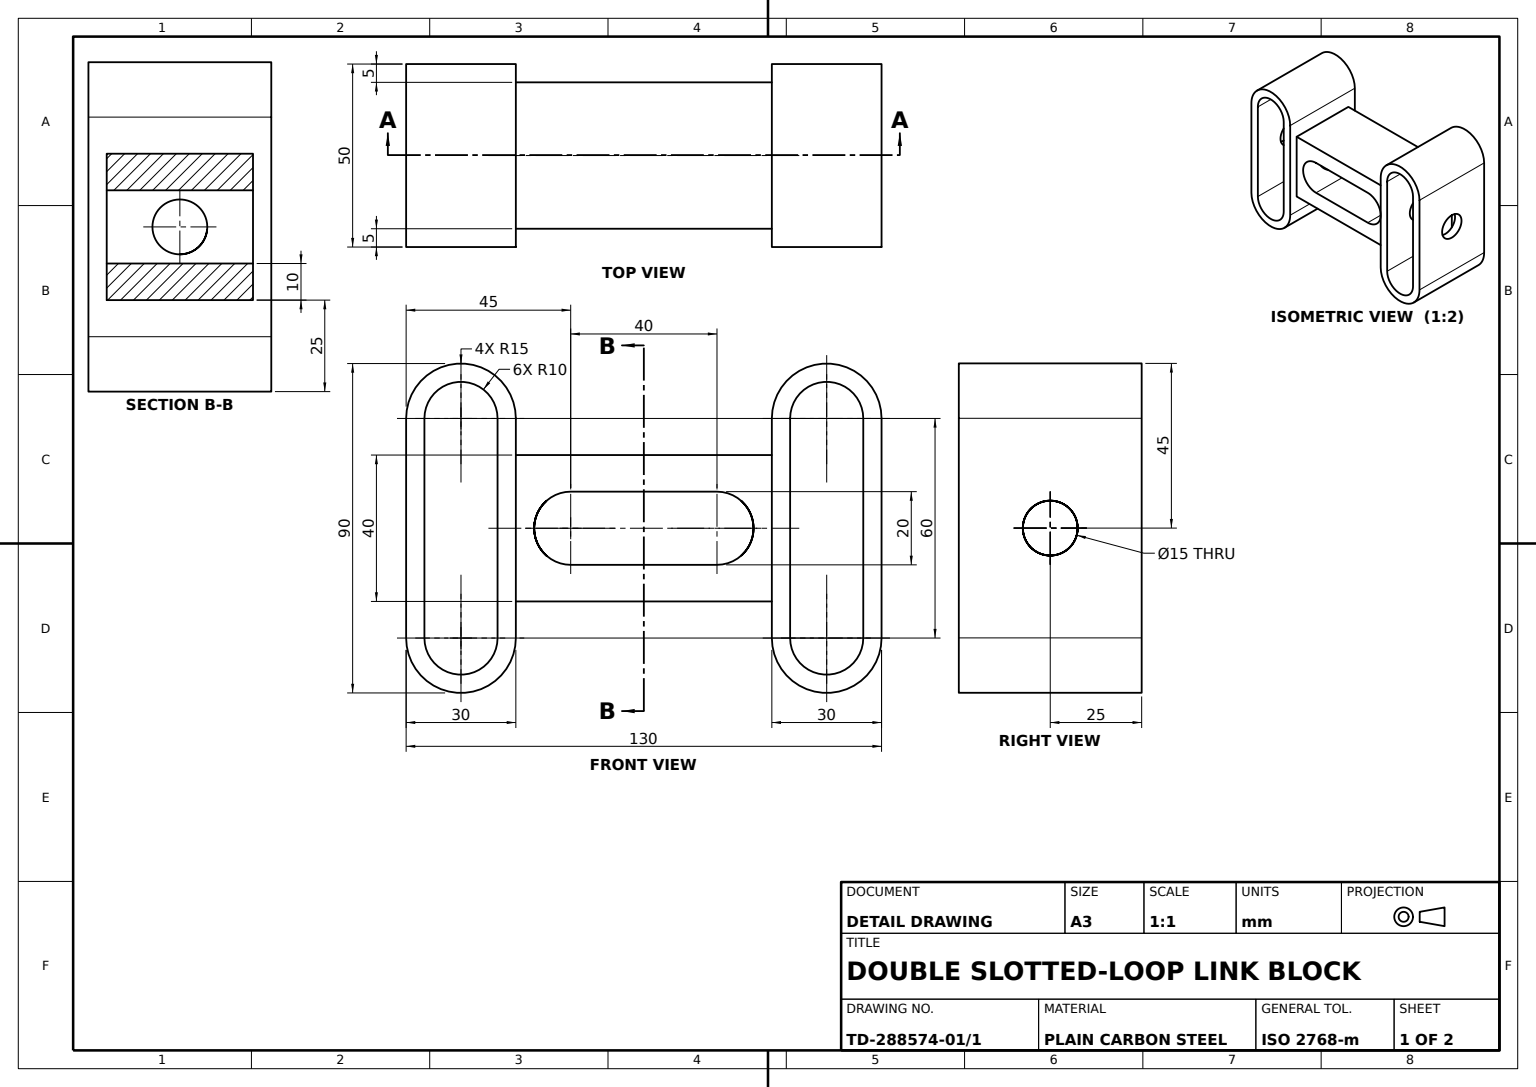
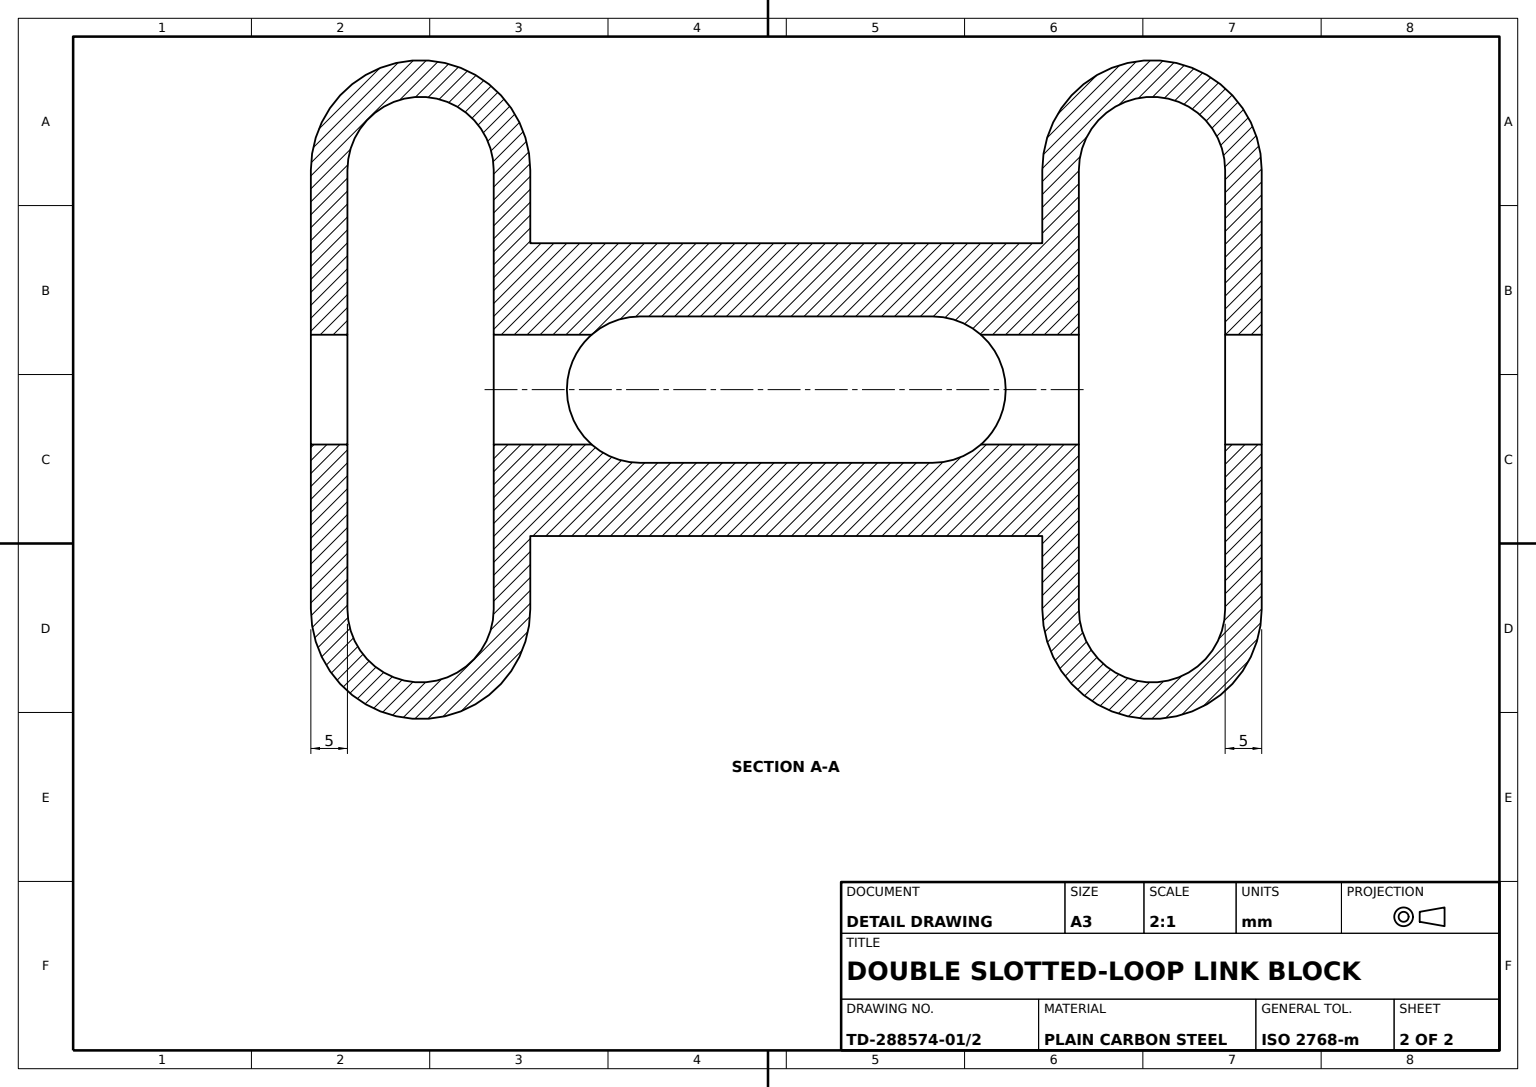
from build123d import *

# Parameters (mm, degrees)
END_PLATES_DEPTH     = 50
END_PLATES_2_DEPTH   = 50
CENTRE_WEB_PROFILE_W = 70
CENTRE_WEB_PROFILE_H = 40
CENTRE_WEB_DEPTH     = 20
CROSS_HOLE_SKETCH_R  = 7.5
CROSS_HOLE_DEPTH     = 147.372811683


with BuildPart() as part:
    # End Plates Profile → End Plates (new body)
    with BuildSketch(Plane.XY):
        with BuildLine():
            Line((15, 30), (15, -30))
            ThreePointArc((15, -30), (0, -45), (-15, -30))
            Line((-15, -30), (-15, 30))
            ThreePointArc((-15, 30), (0, 45), (15, 30))
        make_face()
        with BuildLine():
            Line((10, 30), (10, -30))
            ThreePointArc((10, -30), (0, -40), (-10, -30))
            Line((-10, -30), (-10, 30))
            ThreePointArc((-10, 30), (0, 40), (10, 30))
        make_face(mode=Mode.SUBTRACT)
    extrude(amount=END_PLATES_DEPTH)



with BuildPart() as body_2:
    # End Plates Profile → End Plates 2 (new body)
    with BuildSketch(Plane.XY):
        with BuildLine():
            Line((115, 30), (115, -30))
            ThreePointArc((115, -30), (100, -45), (85, -30))
            Line((85, -30), (85, 30))
            ThreePointArc((85, 30), (100, 45), (115, 30))
        make_face()
        with BuildLine():
            Line((110, 30), (110, -30))
            ThreePointArc((110, -30), (100, -40), (90, -30))
            Line((90, -30), (90, 30))
            ThreePointArc((90, 30), (100, 40), (110, 30))
        make_face(mode=Mode.SUBTRACT)
    extrude(amount=END_PLATES_2_DEPTH)


with BuildPart() as part_1:
    add(part.part)

    add(body_2.part)  # Centre Web merges body 2
    # Centre Web Profile → Centre Web (add, symmetric)
    with BuildSketch(Plane.XY.offset(25)):
        with Locations((50, 0)):
            Rectangle(CENTRE_WEB_PROFILE_W, CENTRE_WEB_PROFILE_H)
        with BuildLine():
            ThreePointArc((70, -10), (80, 0), (70, 10))
            Line((70, 10), (30, 10))
            ThreePointArc((30, 10), (20, 0), (30, -10))
            Line((30, -10), (70, -10))
        make_face(mode=Mode.SUBTRACT)
    extrude(amount=CENTRE_WEB_DEPTH, both=True)

    # Cross Hole Sketch → Cross Hole (cut, through all)
    with BuildSketch(Plane.ZY.offset(15)):
        with Locations(Location((25, 0, 0), (0, 0, 270))):
            Circle(CROSS_HOLE_SKETCH_R)
    extrude(amount=-CROSS_HOLE_DEPTH, mode=Mode.SUBTRACT)


solid = part_1.part
